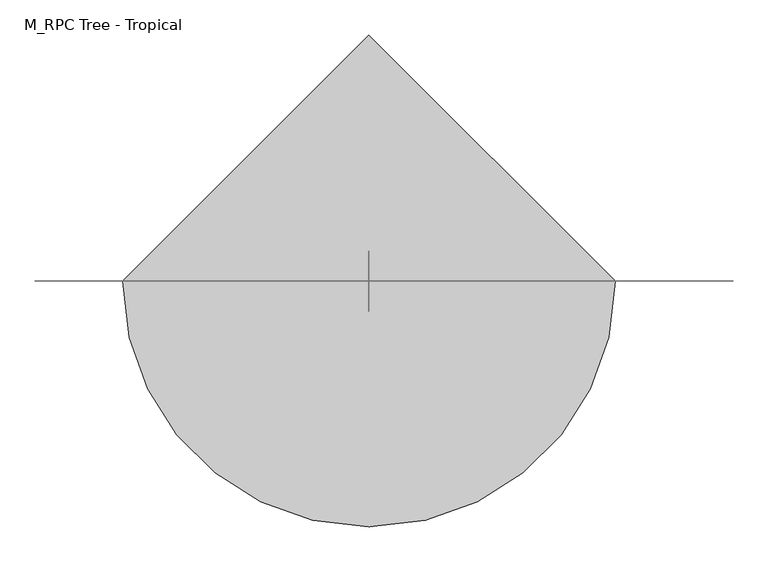
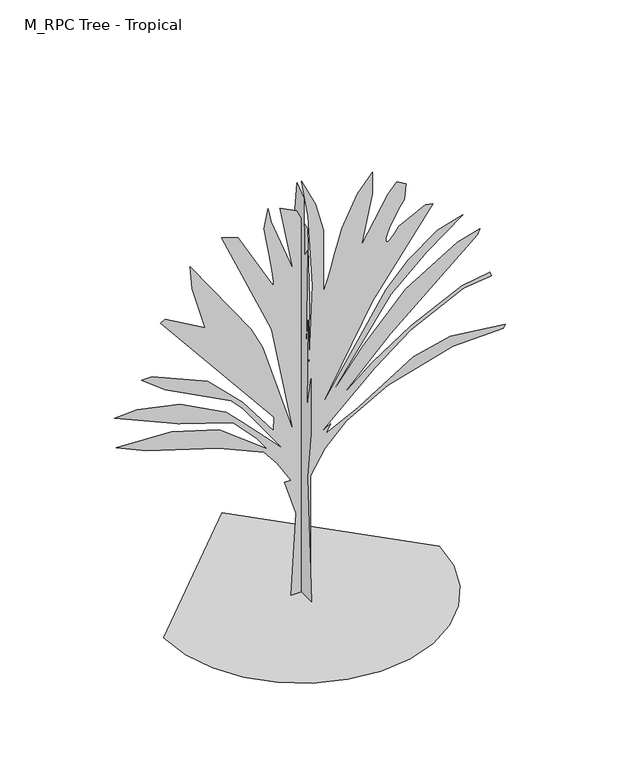
"""IFC4 building model written with IfcOpenShell, lengths in millimetres: geographic element geometry, M_RPC Tree - Tropical."""

from ifc_helpers import new_model, si_unit, origin, place, context, project, spatial, triangles, source, transform, mapped, element, save


def m_rpc_tree_tropical_44340318(model_context):
    return source(origin(), model_context, "Body", "Tessellation", [
        triangles([(-92.0803806, -0.0077972, 0.060482), (-46.9646024, -0.0078429, 766.967938), (-152.2349211, -0.0078626, 1097.8156214), (-92.0803806, -0.0078623, 1092.8031366), (-217.401701, -0.0078745, 1298.3307804), (-337.7109999, -0.0078835, 1448.7157871), (-743.7512592, -0.007894, 1624.165979), (-1395.4241272, -0.0079062, 1829.6935501), (-1666.1167614, -0.0079137, 1955.0136623), (-1164.8315163, -0.0079122, 1929.9486225), (-738.7387745, -0.0079044, 1799.6160255), (-307.6334753, -0.0078847, 1468.7658714), (-402.8785337, -0.0078928, 1604.1134239), (-613.4187349, -0.0079059, 1824.6784492), (-1104.6764671, -0.0079155, 1985.0910416), (-1681.1568317, -0.0079307, 2240.7462215), (-1475.6291153, -0.0079313, 2250.7738071), (-1089.6389402, -0.0079262, 2165.5537182), (-678.5837254, -0.0079131, 1944.9885475), (-538.2236155, -0.0079047, 1804.6285103), (-167.2734381, -0.007882, 1423.6507473), (-523.1861249, -0.0079119, 1924.9361378), (-633.4686739, -0.0079188, 2040.233606), (-1224.9865654, -0.0079373, 2351.0288795), (-1435.5266212, -0.0079472, 2516.4513405), (-1340.2815628, -0.0079472, 2516.4513405), (-844.0088024, -0.007934, 2295.8887859), (-528.1986096, -0.0079158, 1990.1036716), (-252.4909836, -0.0078937, 1619.1533489), (-247.4789712, -0.0079014, 1749.4859459), (-1265.0890594, -0.0079758, 2997.6766182), (-1224.9865654, -0.0079773, 3022.7518318), (-864.0613575, -0.0079648, 2812.2016022), (-984.3689123, -0.0079896, 3228.2767868), (-999.40891, -0.0080021, 3438.8270164), (-453.0060699, -0.0079555, 2656.8014946), (-347.7360057, -0.007943, 2446.273938), (-72.0293698, -0.0078895, 1548.9733303), (-267.5309813, -0.0079516, 2591.6514015), (-718.6887629, -0.0080129, 3619.2770485), (-568.30114, -0.0080096, 3564.1519249), (-257.5059754, -0.0079764, 3007.7015877), (-249.5834757, -0.0079763, 3005.2767357), (-250.6059787, -0.0079784, 3040.9765915), (-259.0834773, -0.0079824, 3108.4768318), (-273.5234934, -0.007988, 3201.3766846), (-292.4334947, -0.0079947, 3313.376825), (-314.325981, -0.0080021, 3438.0770622), (-337.7109999, -0.0080099, 3569.1519104), (-297.6085058, -0.0080204, 3744.6019569), (-272.5434842, -0.0080126, 3614.277063), (-77.0418727, -0.0079815, 3092.9266182), (-192.3376967, -0.0080186, 3714.5270485), (-41.9520995, -0.0080141, 3639.3269875), (53.2924502, -0.0080018, 3433.8020325), (73.3437154, -0.0079612, 2752.0514946), (63.3179556, -0.0079164, 2000.1286411), (98.4077288, -0.007969, 2882.4016777), (58.3052029, -0.008009, 3554.1269554), (3.1637226, -0.0080296, 3900.0020645), (128.4849899, -0.0080141, 3639.3269875), (198.6650176, -0.0079979, 3368.6519394), (198.6650176, -0.0079636, 2792.1516632), (203.4877792, -0.0079638, 2795.8264389), (216.9920421, -0.007966, 2833.1764847), (237.730293, -0.0079699, 2898.5765625), (264.256817, -0.0079752, 2986.4267235), (295.1218298, -0.0079814, 3091.1017296), (328.8818513, -0.0079883, 3207.0269211), (364.089368, -0.0079956, 3328.5267723), (504.4494779, -0.0080123, 3609.252079), (639.796994, -0.0080216, 3764.6521866), (639.796994, -0.0080096, 3564.1519249), (539.5394872, -0.0079824, 3107.9768623), (780.1571039, -0.008006, 3503.9768188), (860.362092, -0.0080117, 3599.2271095), (940.5671528, -0.0080087, 3549.1019714), (925.5296986, -0.0080003, 3408.7518173), (888.2171505, -0.0079967, 3347.7767601), (852.6171432, -0.0079932, 3288.4518929), (820.4345873, -0.0079898, 3232.3518288), (793.3820961, -0.0079868, 3181.1267578), (773.1695944, -0.0079841, 3136.4018715), (761.5070795, -0.0079819, 3099.7767815), (760.1045488, -0.0079803, 3072.8766792), (766.8870564, -0.0079795, 3058.5516815), (778.1395672, -0.0079794, 3057.1267685), (793.1196121, -0.0079799, 3066.4267822), (811.0821058, -0.007981, 3084.3268524), (831.2796375, -0.0079825, 3108.6768196), (852.9671219, -0.0079842, 3137.326815), (875.3996189, -0.007986, 3168.1266792), (1116.017272, -0.0079932, 3288.4268944), (1181.1848059, -0.0079923, 3273.4019394), (639.796994, -0.0079483, 2536.5012794), (168.5880017, -0.0078976, 1684.3208828), (760.1045488, -0.0079525, 2606.6763565), (960.6197079, -0.0079651, 2817.2265862), (1221.2873726, -0.0079764, 3007.7015877), (1451.8799835, -0.0079806, 3077.9016632), (1131.0572697, -0.0079663, 2837.2765251), (805.2220711, -0.0079489, 2546.5265396), (243.7807958, -0.0079014, 1749.4859459), (559.5920059, -0.0079253, 2150.516264), (935.554668, -0.0079492, 2551.5515236), (1401.7499039, -0.007966, 2832.2515411), (1607.277475, -0.0079693, 2887.4016632), (1582.2125805, -0.0079666, 2842.3015091), (800.2071156, -0.0079268, 2175.5786877), (364.089368, -0.0079008, 1739.4609764), (639.796994, -0.007914, 1960.0261471), (985.684675, -0.0079274, 2185.6062733), (1441.8523979, -0.0079406, 2406.1712986), (1697.5100487, -0.007943, 2446.273938), (1707.5351635, -0.0079406, 2406.1712986), (1456.8924683, -0.0079388, 2376.093774), (985.684675, -0.007925, 2145.5036339), (659.8470057, -0.0079104, 1899.8735687), (178.6137706, -0.0078838, 1453.7282719), (263.8318066, -0.0078871, 1508.8708363), (223.7295306, -0.0078823, 1428.663232), (514.4744837, -0.007891, 1574.0358994), (1005.7346867, -0.0079095, 1884.8334984), (1341.5973255, -0.007914, 1960.0261471), (1832.8576012, -0.0079107, 1904.8860535), (1817.8176762, -0.0079086, 1869.7960442), (1361.6474098, -0.007908, 1859.7686039), (780.1571039, -0.0078979, 1689.3335129), (404.1918983, -0.0078856, 1483.8057964), (213.7037799, -0.0078742, 1293.3156796), (83.3694661, -0.0078614, 1077.763139), (83.3694661, -0.0077972, 0.0), (0.2420326, 53.1400295, 0.0511), (0.2420216, -154.4255849, 0.0510875), (0.2420326, -96.0480527, 1148.1506304), (0.2420216, -147.93958, 1595.715826), (0.2420216, -147.9393348, 2114.631245), (0.2420326, -89.5615482, 1803.2810635), (0.2420326, -102.5340576, 2646.5265404), (0.2420326, -70.1020392, 2341.6563412), (0.2420326, -96.0480527, 3301.6519592), (0.2420326, -50.64278, 3223.8017693), (0.2420326, -44.1565253, 3768.6772316), (0.2420433, 66.1132883, 3846.5021324), (0.2420433, 130.9775703, 3321.1019348), (0.2420433, 150.4368386, 2568.6763504), (0.2420433, 105.0318066, 1920.0386169), (0.2420326, 53.1400295, 1102.7456257), (-1239.0439922, 0.0, 0.0566583), (-1206.2815298, -283.9526533, 0.0566415), (-1112.9764692, -544.7152977, 0.056626), (-966.6013922, -774.8229092, 0.0566123), (-774.6262642, -966.7980371, 0.0566008), (-544.5186164, -1113.1731142, 0.056592), (-283.7559902, -1206.4781748, 0.0565865), (0.1967145, -1239.2406372, 0.0565845), (284.1493165, -1206.4781748, 0.0565865), (544.911979, -1113.1731142, 0.056592), (775.0195541, -966.7980371, 0.0566008), (966.9946821, -774.8229092, 0.0566123), (1113.3697592, -544.7152977, 0.056626), (1206.6748198, -283.9526533, 0.0566415), (1239.4372822, 0.0001083, 0.0566583), (0.1964973, 1239.2406372, 0.0567323)], [[59, 60, 61], [99, 100, 101], [8, 9, 10], [49, 50, 51], [98, 99, 101], [15, 16, 17], [15, 17, 18], [119, 120, 121], [34, 35, 36], [33, 34, 36], [98, 101, 102], [97, 98, 102], [24, 25, 26], [24, 26, 27], [23, 24, 27], [23, 27, 28], [22, 23, 28], [22, 28, 29], [21, 22, 29], [7, 8, 10], [7, 10, 11], [71, 72, 73], [106, 107, 108], [106, 108, 109], [105, 106, 109], [104, 105, 109], [104, 109, 110], [103, 104, 110], [39, 40, 41], [39, 41, 42], [52, 53, 54], [52, 54, 55], [52, 55, 56], [59, 61, 62], [58, 59, 62], [58, 62, 63], [57, 58, 63], [7, 11, 12], [6, 7, 12], [15, 18, 19], [14, 15, 19], [14, 19, 20], [13, 14, 20], [13, 20, 21], [12, 13, 21], [93, 94, 95], [92, 93, 95], [91, 92, 95], [90, 91, 95], [89, 90, 95], [88, 89, 95], [87, 88, 95], [2, 3, 4], [96, 97, 102], [96, 102, 103], [124, 125, 126], [124, 126, 127], [39, 42, 43], [49, 51, 52], [48, 49, 52], [47, 48, 52], [46, 47, 52], [45, 46, 52], [44, 45, 52], [86, 87, 95], [114, 115, 116], [113, 114, 116], [30, 31, 32], [30, 32, 33], [30, 33, 36], [30, 36, 37], [30, 37, 38], [29, 30, 38], [21, 29, 38], [131, 132, 1], [131, 1, 2], [131, 2, 4], [5, 6, 12], [5, 12, 21], [123, 124, 127], [123, 127, 128], [122, 123, 128], [122, 128, 129], [121, 122, 129], [121, 129, 130], [113, 116, 117], [112, 113, 117], [111, 112, 117], [111, 117, 118], [110, 111, 118], [110, 118, 119], [103, 110, 119], [96, 103, 119], [71, 73, 74], [70, 71, 74], [69, 70, 74], [68, 69, 74], [44, 52, 56], [43, 44, 56], [39, 43, 56], [39, 56, 57], [38, 39, 57], [75, 76, 77], [75, 77, 78], [74, 75, 78], [74, 78, 79], [74, 79, 80], [74, 80, 81], [74, 81, 82], [74, 82, 83], [74, 83, 84], [74, 84, 85], [67, 68, 74], [119, 121, 130], [130, 131, 4], [130, 4, 5], [130, 5, 21], [119, 130, 21], [119, 21, 38], [96, 119, 38], [96, 38, 57], [95, 96, 57], [95, 57, 63], [95, 63, 64], [86, 95, 64], [86, 64, 65], [86, 65, 66], [86, 66, 67], [86, 67, 74], [86, 74, 85], [138, 139, 140], [136, 137, 138], [140, 141, 142], [143, 144, 145], [142, 143, 145], [142, 145, 146], [140, 142, 146], [140, 146, 147], [138, 140, 147], [138, 147, 148], [136, 138, 148], [135, 136, 148], [134, 135, 148], [134, 148, 133], [163, 164, 149], [162, 163, 149], [162, 149, 150], [161, 162, 150], [161, 150, 151], [161, 151, 152], [160, 161, 152], [159, 160, 152], [159, 152, 153], [159, 153, 154], [159, 154, 155], [159, 155, 156], [159, 156, 157], [159, 157, 158]], closed=False),
    ])


if __name__ == "__main__":
    model = new_model("IFC4")
    model_context = context("Model", 3, world=origin())
    ifc_project = project(units=[si_unit("LENGTHUNIT", "METRE", prefix="MILLI")], contexts=[model_context])
    site = spatial("IfcSite", under=ifc_project)
    building = spatial("IfcBuilding", under=site)
    placement = place(None, origin())
    m_rpc_tree_tropical_shape = m_rpc_tree_tropical_44340318(model_context)
    element("IfcGeographicElement", 1, ObjectType="M_RPC Tree - Tropical", at=placement, inside=building, context=model_context, shape_type="MappedRepresentation", body=[
        mapped(m_rpc_tree_tropical_shape, transform((0.0, 0.0, 0.0), x_axis=(1.0, 0.0, 0.0), y_axis=(0.0, 1.0, 0.0), z_axis=(0.0, 0.0, 1.0))),
    ])
    save(model, "model.ifc")

# Revit data of these elements
# Type "M_RPC Tree - Tropical"
#   built-in parameter 1005198 = "{2, 15},{39, RPC-16-G2M6-EAFX-C5H6-W000-ST1L-LVER-AU},{1, 0},{1, 0},{2, 35},{1, 8},{5, Color},{1, 0},{1, 0},{3, 0.8},{3, 0.8},{3, 0.8},{1, 8},{7, BBoxMin},{1, 0},{1, 0},{1, 0},{1, 0},{1, 0},{1, 8},{7, BBoxMax},{1, 0},{1, 0},{1, 0},{1, 0},{1, 0},{2, 11},{9, RPCTypeId},{1, 0},{1, 0},{39, RPC-16-G2M6-EAFX-C5H6-W000-ST1L-LVER-AU},{1, 6},{14, RPCPlantHeight},{1, 0},{1, 0},{7, 12.7953},{2, 11},{7, keyword},{1, 0},{1, 0},{74, :Geometry:RPC:Traveler's Palm:Ravenala madagascariensis:fan:palm:tropical.},{2, 11},{8, category},{1, 0},{1, 0},{17, :Trees [Tropical]},{2, 11},{12, LocalizedUID},{1, 0},{1, 0},{15, Traveler's Palm},{2, 14},{6, Height},{1, 0},{1, 0},{7, 12.7953},{1, 2},{16, Cast Reflections},{1, 0},{1, 0},{1, 0},{1, 2},{12, Cast Shadows},{1, 0},{1, 0},{1, 1},{1, 2},{9, Lock View},{1, 0},{1, 0},{1, 0},{1, 4},{5, ViewC},{1, 0},{1, 0},{1, 0},{2, 11},{20, AdvancedUIDefinition},{1, 0},{1, 0},{0, },{2, 11},{10, AssetLibID},{1, 0},{1, 0},{36, 4D3F6E72-3F99-4203-98E9-AF80B3C7A7A4},{2, 11},{10, BaseSchema},{1, 0},{1, 0},{9, RPCSchema},{2, 11},{12, ExchangeGUID},{1, 0},{1, 0},{0, },{1, 2},{6, Hidden},{1, 0},{1, 0},{1, 0},{1, 4},{11, RPCCategory},{1, 0},{1, 0},{1, 0},{2, 11},{8, RPCImage},{1, 0},{1, 0},{0, },{1, 4},{13, SchemaVersion},{1, 0},{1, 0},{1, 4},{2, 11},{12, UIDefinition},{1, 0},{1, 0},{0, },{2, 11},{6, UIName},{1, 0},{1, 0},{39, RPC-16-G2M6-EAFX-C5H6-W000-ST1L-LVER-AU},{2, 11},{11, VersionGUID},{1, 0},{1, 0},{9, RPCSchema},{2, 11},{9, assettype},{1, 0},{1, 0},{11, RPCGeometry},{2, 11},{11, description},{1, 0},{1, 0},{0, },{2, 11},{9, localname},{1, 0},{1, 0},{3, RPC},{2, 11},{9, localtype},{1, 0},{1, 0},{3, RPC},{1, 4},{8, revision},{1, 0},{1, 0},{1, 1},{2, 11},{9, thumbnail},{1, 0},{1, 0},{0, },{1, 4},{7, version},{1, 0},{1, 0},{1, 1},{1, 2},{20, RPC_Cast Reflections},{1, 0},{1, 0},{1, 1},{1, 2},{16, RPC_Cast Shadows},{1, 0},{1, 0},{1, 1},{1, 2},{13, RPC_Lock View},{1, 0},{1, 0},{1, 0},{1, 4},{9, RPC_ViewC},{1, 0},{1, 0},{1, 0},{21, assetlibrary_base.fbx},{1, 5},"
#   built-in parameter 1005195 = "RPC-16-G2M6-EAFX-C5H6-W000-ST1L-LVER-AU"
#   Height = 3900 mm
#   Plan Symbol = element 405753
#   Description = (empty or 0)
#   Default Elevation = 0
